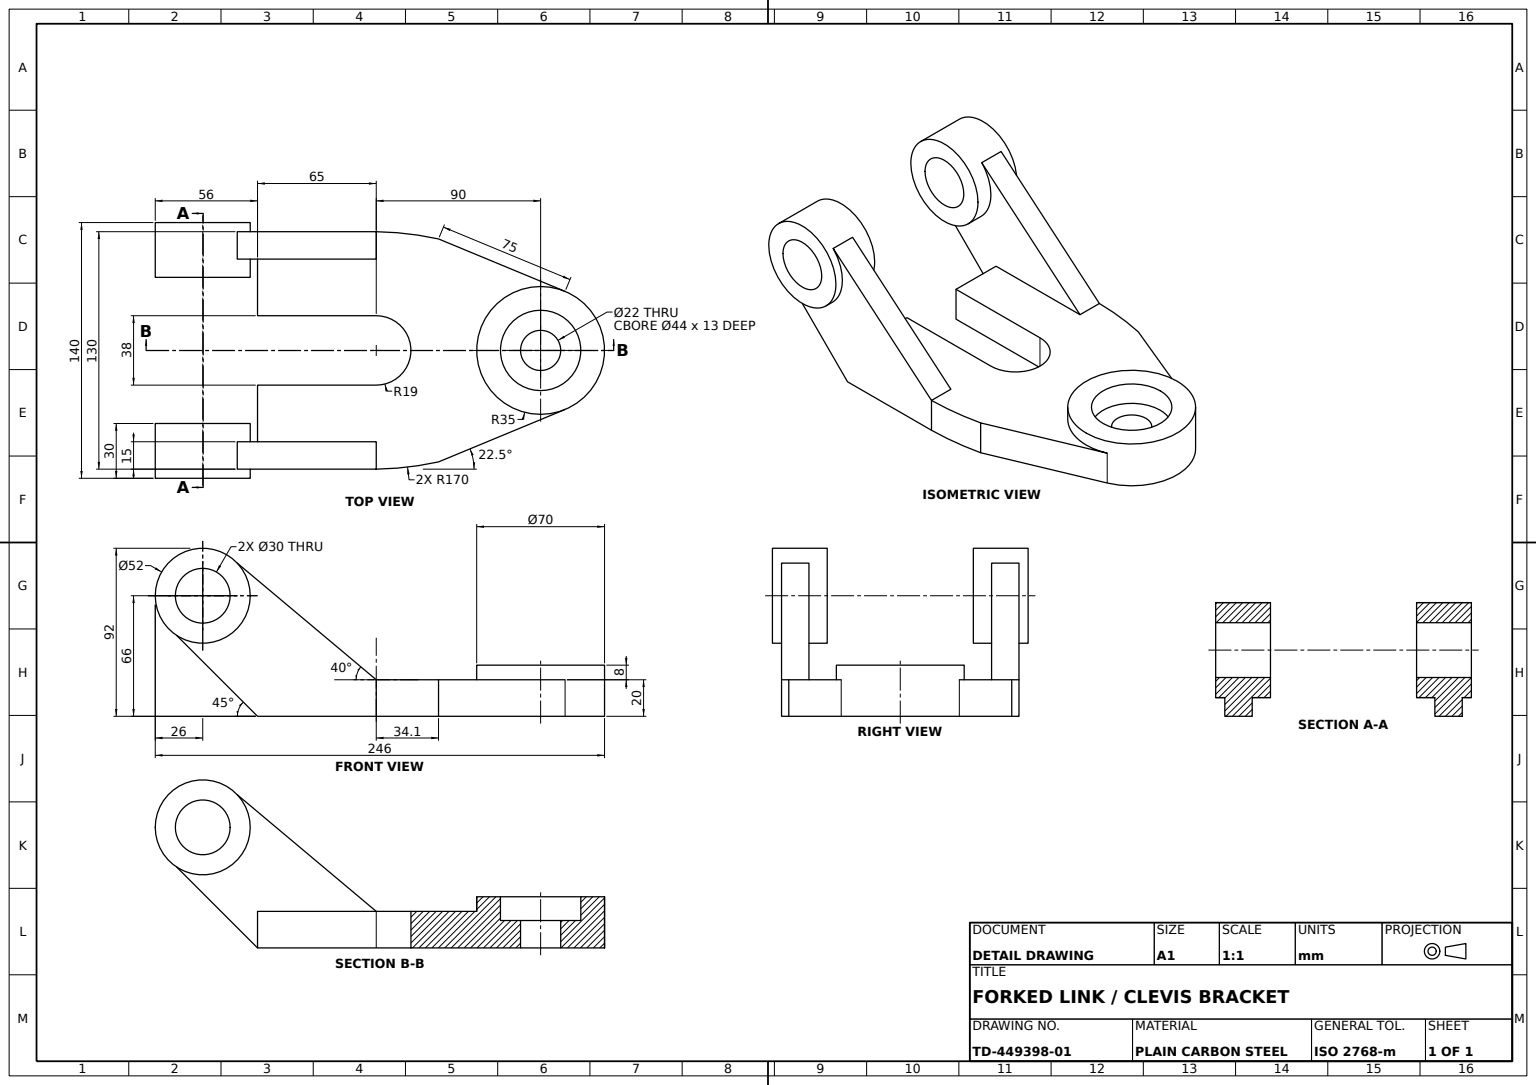
SolidWorks part; units mm, degrees
material "Plain Carbon Steel"
ref_plane "Front Plane" through (0, 0, 0) normal (0, 0, 1) x (1, 0, 0)
ref_plane "Top Plane" through (0, 0, 0) normal (0, 1, 0) x (1, 0, 0)
ref_plane "Right Plane" through (0, 0, 0) normal (1, 0, 0) x (0, 0, -1)
sketch "Base Plate Sketch" plane through (0, 0, 0) normal (0, 1, 0) x (1, 0, 0)
  line L0 (0, 0) -> (0, 46)
  line L1 (0, 46) -> (65, 46)
  line L2 (0, 0) -> (65, 0)
  line L3 (168.3939, 13.3358) -> (99.103, 42.037)
  line L4 (65, -38) -> (0, -38)
  line L5 (0, -38) -> (0, -84)
  line L6 (0, -84) -> (65, -84)
  line L8 (168.3939, -51.3358) -> (99.103, -80.037)
  arc A0 (168.3939, -51.3358) -> (168.3939, 13.3358) centre (155, -19) ccw
  arc A1 (65, -38) -> (65, 0) centre (65, -19) ccw
  arc A2 (65, 46) -> (99.103, 42.037) centre (62.5288, -123.982) cw
  arc A3 (65, -84) -> (99.103, -80.037) centre (62.5288, 85.982) ccw
  dimension "D6" = 70
  dimension "D8" = 19
  dimension "D14" = 170
  dimension "D16" = 170
  dimension "D1" = 46
  dimension "D2" = 65
  dimension "D3" = 38
  dimension "D4" = 46
  dimension "D5" = 65
  dimension "D7" = 90
  dimension "D9" = 19
  dimension "D10" = 45
  dimension "D11" = 55.897
  dimension "D12" = 75
  dimension "D13" = 75
  dimension "D15" = 65
extrude "Base Plate" add sketch "Base Plate Sketch" along normal blind 20
sketch "Pivot Boss Sketch" plane through (0, 20, 0) normal (0, 1, 0) x (1, 0, 0)
  circle A0 centre (155, -19) radius 35
  dimension "D1" = 70
extrude "Pivot Boss Ø70" add sketch "Pivot Boss Sketch" along normal blind 8
sketch "Arm Web 1 Sketch" plane through (0, 0, 84) normal (0, 0, 1) x (1, 0, 0)
  line L0 (65, 20) -> (65, 0) construction
  line L1 (0, 0) -> (-44.2583, 44.2583)
  line L2 (65, 20) -> (-11.1036, 83.8585)
  line L3 (0, 0) -> (65, 0)
  line L4 (65, 0) -> (65, 20)
  arc A0 (-11.1036, 83.8585) -> (-44.2583, 44.2583) centre (-30, 66) ccw
  dimension "D3" = 52
  dimension "D1" = 76.1036
  dimension "D2" = 109.2583
  dimension "D4" = 66
  dimension "D5" = 30
extrude "Arm Web 1" add sketch "Arm Web 1 Sketch" against normal blind 15
sketch "Arm Web 2 Sketch" plane through (0, 0, -46) normal (0, 0, -1) x (-1, 0, 0)
  line L0 (-65, 20) -> (-65, 0)
  line L1 (0, 0) -> (44.2583, 44.2583)
  line L2 (-65, 20) -> (11.1036, 83.8585)
  line L3 (-65, 0) -> (0, 0)
  arc A0 (44.2583, 44.2583) -> (11.1036, 83.8585) centre (30, 66) ccw
extrude "Arm Web 2" add sketch "Arm Web 2 Sketch" against normal blind 15
ref_plane "Plane1" through (0, 0, -51) normal (0, 0, 1) x (1, 0, 0)
sketch "Lug Boss 1 Sketch" plane through (0, 0, -51) normal (0, 0, 1) x (1, 0, 0)
  circle A0 centre (-30, 66) radius 26
  dimension "D1" = 52
extrude "Lug Boss 1 Ø52" add sketch "Lug Boss 1 Sketch" along normal blind 30
ref_plane "Plane2" through (0, 0, 89) normal (0, 0, 1) x (1, 0, 0)
sketch "Lug Boss 2 Sketch" plane through (0, 0, 89) normal (0, 0, 1) x (1, 0, 0)
  circle A0 centre (-30, 66) radius 26
  dimension "D1" = 52
extrude "Lug Boss 2 Ø52" add sketch "Lug Boss 2 Sketch" against normal blind 30
sketch "Lug Bore Sketch" plane through (0, 0, 89) normal (0, 0, 1) x (1, 0, 0)
  circle A0 centre (-30, 66) radius 15
  dimension "D1" = 30
extrude "Lug Bore Ø30" cut sketch "Lug Bore Sketch" against normal through all
sketch "Pivot Counterbore Sketch" plane through (0, 28, 0) normal (0, 1, 0) x (1, 0, 0)
  circle A0 centre (155, -19) radius 22
  dimension "D1" = 44
extrude "Pivot Counterbore Ø44" cut sketch "Pivot Counterbore Sketch" against normal blind 13
sketch "Pivot Hole Sketch" plane through (0, 15, 0) normal (0, 1, 0) x (1, 0, 0)
  circle A0 centre (155, -19) radius 11
  dimension "D1" = 22
extrude "Pivot Hole Ø22" cut sketch "Pivot Hole Sketch" against normal through all
